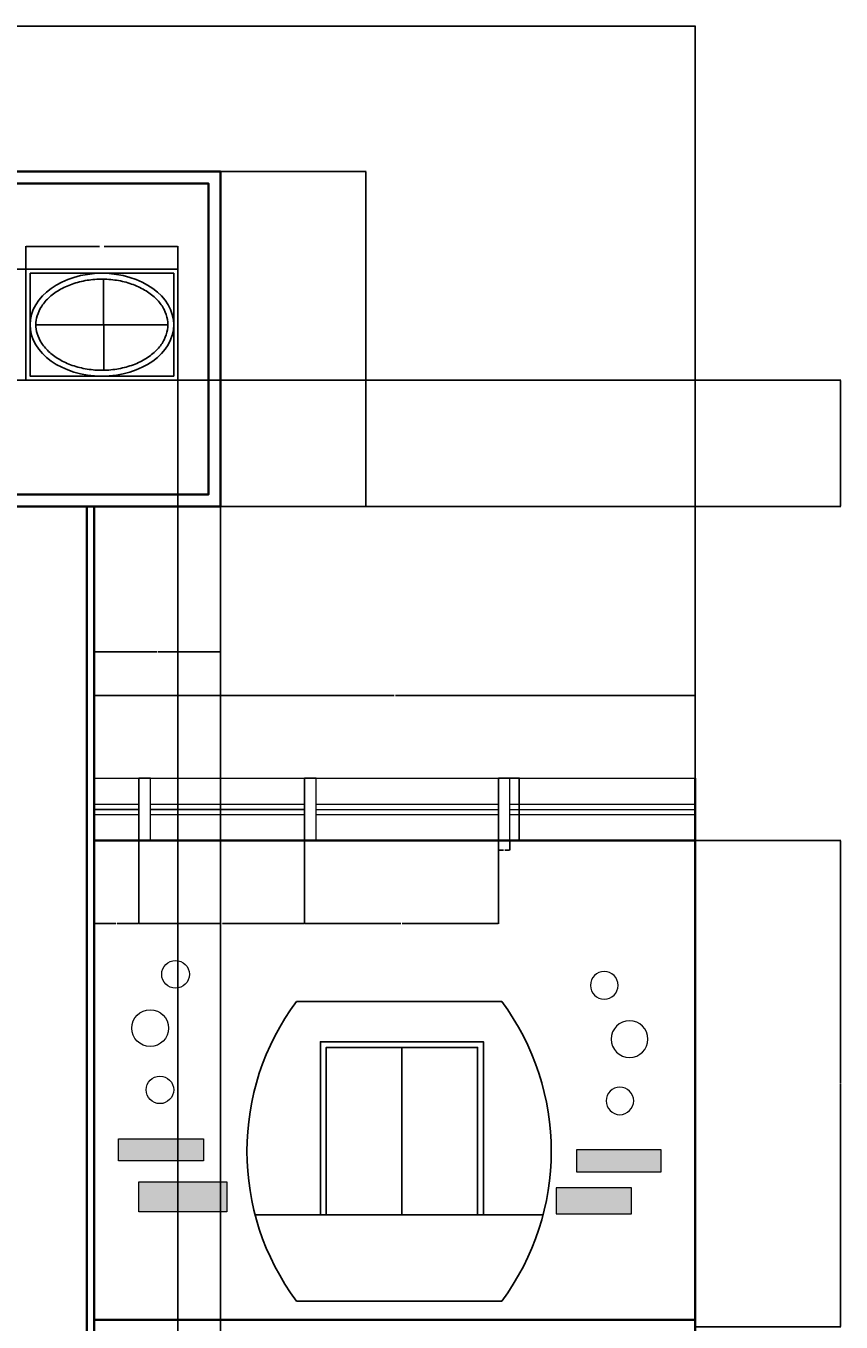
# Model space of a CAD drawing. Units: inches. Extents: x 328 to 2318, y 647 to 2548.
# Tile 5 of 5: x 1799 to 2318, y 1724 to 2548. Entities that reach past the tile are written whole.
import ezdxf

# ---------------------------------------------------------------- set-up
doc = ezdxf.new("R2010")
doc.units = ezdxf.units.IN
doc.header["$MEASUREMENT"] = 0
for name, color, linetype, lineweight in [('A-ANNO-DIMS', 2, 'Continuous', 18), ('A-ELEV', 7, 'Continuous', 35), ('A-ELEV-ORNM', 7, 'Continuous', 18), ('A-GLAZ', 4, 'Continuous', 25), ('A-ROOF', 7, 'Continuous', 35), ('A-ROOF-HRAL', 8, 'Continuous', 18)]:
    doc.layers.add(name, color=color, linetype=linetype, lineweight=lineweight)
doc.layers.add('A-ELEV-ORNM-PATT', color=18, linetype='Continuous', lineweight=13, true_color=0x000000)
doc.styles.get("Standard").update_dxf_attribs({"font": 'arial.ttf'})
doc.dimstyles.get("Standard").update_dxf_attribs({"dimtxt": 0.18, "dimasz": 0.18, "dimexe": 0.18, "dimexo": 0.0625, "dimgap": 0.09, "dimtad": 0, "dimtih": 1, "dimtoh": 1, "dimdec": 4, "dimzin": 0, "dimdsep": 46, "dimtxsty": 'Standard', "dimcen": 0.09, "dimadec": 0, "dimazin": 0, "dimtfac": 1, "dimtdec": 4, "dimtofl": 0, "dimtmove": 0, "dimatfit": 3, "dimfxl": 1, "dimtolj": 1, "dimtzin": 0, "dimarcsym": 0})

# ---------------------------------------------------------------- blocks, each defined once
blk = doc.blocks.new('WIN-ELEV-CURVED-SURROUND')
for p, q in [((162.11, 190.69), (31.57, 190.69)), ((98.64, 161.37), (98.64, 54.8)), ((5.23, 54.8), (188.45, 54.8)), ((31.57, 0), (162.11, 0))]:
    blk.add_line(p, q)
for points in [[(150.48, 54.8), (150.48, 165.07), (46.8, 165.07), (46.8, 54.8)], [(146.78, 54.8), (146.78, 161.37), (50.49, 161.37), (50.49, 54.8)]]:
    blk.add_lwpolyline(points)
for centre, start, end in [((159.76, 95.35), 143.35881, 216.64119), ((33.92, 95.35), 323.35881, 36.64119)]:
    blk.add_arc(centre, 159.76, start, end)
blk = doc.blocks.new('WIN-ELEV-OVAL')
for p, q in [((49.54, 6.37), (49.37, 64.33)), ((6.36, 35.36), (90.36, 35.36))]:
    blk.add_line(p, q)
for points in [[(0, 70.7), (96.72, 70.7), (96.72, 0), (0, 0)], [(2.67, 68.03), (94.06, 68.03), (94.06, 2.67), (2.67, 2.67)]]:
    blk.add_lwpolyline(points, close=True)
blk.add_ellipse((48.36, 35.35), major_axis=(-45.7, 0), ratio=0.715242)
blk.add_open_spline([(6.36, 35.35), (6.36, 33.47), (6.63, 31.58), (7.79, 27.59), (8.77, 25.48), (11.44, 21.43), (13.14, 19.48), (17.17, 15.88), (19.51, 14.22), (24.72, 11.33), (27.59, 10.09), (33.68, 8.11), (36.9, 7.38), (43.51, 6.46), (46.9, 6.28), (53.63, 6.5), (56.98, 6.89), (63.44, 8.21), (66.55, 9.15), (72.35, 11.49), (75.04, 12.9), (79.83, 16.09), (81.94, 17.87), (85.48, 21.67), (86.9, 23.7), (89.04, 27.86), (89.75, 29.99), (90.45, 34.29), (90.45, 36.45), (89.74, 40.75), (89.02, 42.88), (86.88, 47.04), (85.45, 49.06), (81.9, 52.86), (79.79, 54.64), (74.99, 57.83), (72.3, 59.23), (66.49, 61.57), (63.38, 62.5), (56.92, 63.82), (53.57, 64.21), (46.83, 64.41), (43.45, 64.23), (36.84, 63.31), (33.62, 62.57), (27.53, 60.59), (24.67, 59.35), (19.47, 56.45), (17.13, 54.79), (13.1, 51.18), (11.41, 49.23), (8.75, 45.18), (7.78, 43.07), (6.63, 39.09), (6.36, 37.22), (6.36, 35.35)], degree=3, knots=[0, 0, 0, 0, 0.205219, 0.205219, 0.440189, 0.440189, 0.675159, 0.675159, 0.910128, 0.910128, 1.145098, 1.145098, 1.380068, 1.380068, 1.615038, 1.615038, 1.850008, 1.850008, 2.084978, 2.084978, 2.319948, 2.319948, 2.554918, 2.554918, 2.789887, 2.789887, 3.024857, 3.024857, 3.259827, 3.259827, 3.494797, 3.494797, 3.729767, 3.729767, 3.964737, 3.964737, 4.199707, 4.199707, 4.434676, 4.434676, 4.669646, 4.669646, 4.904616, 4.904616, 5.139586, 5.139586, 5.374556, 5.374556, 5.609526, 5.609526, 5.844496, 5.844496, 6.079466, 6.079466, 6.283185, 6.283185, 6.283185, 6.283185])
blk = doc.blocks.new('FACADE-THREE-ROUNDELS')
for centre, radius in [((27.83, 82.27), 8.8), ((11.7, 48.09), 11.7), ((17.88, 8.77), 8.77)]:
    blk.add_circle(centre, radius)
blk = doc.blocks.new('POST-PARAPET')
blk.add_lwpolyline([(0, 0), (7.34, 0), (7.34, 39.76), (0, 39.76)], close=True)
blk = doc.blocks.new('*D7')
at = {"layer": 'A-ANNO-DIMS', "color": 0, "lineweight": -2, "transparency": 16777216}
for p, q in [((1799.05, 2393.5), (1799.05, 2408.12)), ((1799.23, 2407.94), (1845.92, 2407.94)), ((1895.59, 2407.94), (1848.89, 2407.94)), ((1895.77, 2393.5), (1895.77, 2408.12))]:
    blk.add_line(p, q, dxfattribs=at)
at = {"layer": 'A-ANNO-DIMS', "color": 0, "transparency": 16777216}
for points in [[(1799.23, 2407.97), (1799.23, 2407.91), (1799.05, 2407.94)], [(1895.59, 2407.97), (1895.59, 2407.91), (1895.77, 2407.94)]]:
    blk.add_solid(points, dxfattribs=at)
at = {"layer": 'Defpoints', "color": 0, "transparency": 16777216}
for p in [(1895.77, 2407.94), (1799.05, 2393.44), (1895.77, 2393.44)]:
    blk.add_point(p, dxfattribs=at)
at = {"layer": 'A-ANNO-DIMS', "color": 0, "transparency": 16777216, "insert": (1847.41, 2407.94), "char_height": 0.18, "attachment_point": 5}
blk.add_mtext('\\A1;OVAL WINDOW 97 TYP.', dxfattribs=at)
blk = doc.blocks.new('*D8')
at = {"layer": 'A-ANNO-DIMS', "color": 0, "lineweight": -2, "transparency": 16777216}
for p, q in [((1798.98, 2393.44), (1784.36, 2393.44)), ((1784.54, 2393.26), (1784.54, 2358.27)), ((1784.54, 2322.92), (1784.54, 2357.91)), ((1798.98, 2322.74), (1784.36, 2322.74))]:
    blk.add_line(p, q, dxfattribs=at)
at = {"layer": 'A-ANNO-DIMS', "color": 0, "transparency": 16777216}
for points in [[(1784.51, 2393.26), (1784.57, 2393.26), (1784.54, 2393.44)], [(1784.51, 2322.92), (1784.57, 2322.92), (1784.54, 2322.74)]]:
    blk.add_solid(points, dxfattribs=at)
at = {"layer": 'Defpoints', "color": 0, "transparency": 16777216}
for p in [(1784.54, 2393.44), (1799.05, 2393.44), (1799.05, 2322.74)]:
    blk.add_point(p, dxfattribs=at)
at = {"layer": 'A-ANNO-DIMS', "color": 0, "transparency": 16777216, "insert": (1784.54, 2358.09), "char_height": 0.18, "attachment_point": 5}
blk.add_mtext('\\A1;71 TYP.', dxfattribs=at)
blk = doc.blocks.new('*D9')
at = {"layer": 'A-ANNO-DIMS', "color": 0, "lineweight": -2, "transparency": 16777216}
for p, q in [((2107.09, 2069.59), (2113.17, 2069.59)), ((2112.99, 2069.41), (2112.99, 2049.9)), ((2112.99, 2030.01), (2112.99, 2049.53)), ((2107.09, 2029.83), (2113.17, 2029.83))]:
    blk.add_line(p, q, dxfattribs=at)
at = {"layer": 'A-ANNO-DIMS', "color": 0, "transparency": 16777216}
for points in [[(2112.96, 2069.41), (2113.02, 2069.41), (2112.99, 2069.59)], [(2112.96, 2030.01), (2113.02, 2030.01), (2112.99, 2029.83)]]:
    blk.add_solid(points, dxfattribs=at)
at = {"layer": 'Defpoints', "color": 0, "transparency": 16777216}
for p in [(2107.02, 2069.59), (2112.99, 2069.59), (2107.02, 2029.83)]:
    blk.add_point(p, dxfattribs=at)
at = {"layer": 'A-ANNO-DIMS', "color": 0, "transparency": 16777216, "insert": (2112.99, 2049.71), "char_height": 0.18, "attachment_point": 5}
blk.add_mtext('\\A1;POST 40 TYP.', dxfattribs=at)
blk = doc.blocks.new('*D10')
at = {"layer": 'A-ANNO-DIMS', "color": 0, "lineweight": -2, "transparency": 16777216}
for p, q in [((2099.69, 2029.77), (2099.69, 2023.69)), ((2107.02, 2029.77), (2107.02, 2023.69)), ((2099.87, 2023.87), (2102.9, 2023.87)), ((2106.84, 2023.87), (2103.81, 2023.87))]:
    blk.add_line(p, q, dxfattribs=at)
at = {"layer": 'A-ANNO-DIMS', "color": 0, "transparency": 16777216}
for points in [[(2099.87, 2023.9), (2099.87, 2023.84), (2099.69, 2023.87)], [(2106.84, 2023.9), (2106.84, 2023.84), (2107.02, 2023.87)]]:
    blk.add_solid(points, dxfattribs=at)
at = {"layer": 'Defpoints', "color": 0, "transparency": 16777216}
for p in [(2099.69, 2029.83), (2107.02, 2029.83), (2107.02, 2023.87)]:
    blk.add_point(p, dxfattribs=at)
at = {"layer": 'A-ANNO-DIMS', "color": 0, "transparency": 16777216, "insert": (2103.35, 2023.87), "char_height": 0.18, "attachment_point": 5}
blk.add_mtext('\\A1;7 TYP.', dxfattribs=at)
blk = doc.blocks.new('*D39')
at = {"layer": 'A-ANNO-DIMS', "color": 0, "lineweight": -2, "transparency": 16777216}
for p, q in [((1060.28, 1725.1), (1060.28, 2548.17)), ((2224.98, 2069.65), (2224.98, 2548.17)), ((1060.46, 2547.99), (1642.17, 2547.99)), ((2224.8, 2547.99), (1643.08, 2547.99))]:
    blk.add_line(p, q, dxfattribs=at)
at = {"layer": 'A-ANNO-DIMS', "color": 0, "transparency": 16777216}
for points in [[(1060.46, 2548.02), (1060.46, 2547.96), (1060.28, 2547.99)], [(2224.8, 2548.02), (2224.8, 2547.96), (2224.98, 2547.99)]]:
    blk.add_solid(points, dxfattribs=at)
at = {"layer": 'Defpoints', "color": 0, "transparency": 16777216}
for p in [(2224.98, 2547.99), (2224.98, 2069.59), (1060.28, 1725.04)]:
    blk.add_point(p, dxfattribs=at)
at = {"layer": 'A-ANNO-DIMS', "color": 0, "transparency": 16777216, "insert": (1642.63, 2547.99), "char_height": 0.18, "attachment_point": 5}
blk.add_mtext('\\A1;1164.7', dxfattribs=at)
blk = doc.blocks.new('*D42')
at = {"layer": 'A-ANNO-DIMS', "color": 0, "lineweight": -2, "transparency": 16777216}
for p, q in [((1842.45, 2029.9), (1842.45, 2122.46)), ((1842.63, 2122.28), (2033.32, 2122.28)), ((2224.8, 2122.28), (2034.11, 2122.28)), ((2224.98, 2029.9), (2224.98, 2122.46))]:
    blk.add_line(p, q, dxfattribs=at)
at = {"layer": 'A-ANNO-DIMS', "color": 0, "transparency": 16777216}
for points in [[(1842.63, 2122.31), (1842.63, 2122.25), (1842.45, 2122.28)], [(2224.8, 2122.31), (2224.8, 2122.25), (2224.98, 2122.28)]]:
    blk.add_solid(points, dxfattribs=at)
at = {"layer": 'Defpoints', "color": 0, "transparency": 16777216}
for p in [(2224.98, 2122.28), (1842.45, 2029.83), (2224.98, 2029.83)]:
    blk.add_point(p, dxfattribs=at)
at = {"layer": 'A-ANNO-DIMS', "color": 0, "transparency": 16777216, "insert": (2033.72, 2122.28), "char_height": 0.18, "attachment_point": 5}
blk.add_mtext('\\A1;382.5', dxfattribs=at)
blk = doc.blocks.new('*D46')
at = {"layer": 'A-ANNO-DIMS', "color": 0, "lineweight": -2, "transparency": 16777216}
for p, q in [((2225.04, 2029.83), (2317.61, 2029.83)), ((2317.43, 2029.65), (2317.43, 1875.33)), ((2317.43, 1720.64), (2317.43, 1874.96)), ((2225.04, 1720.46), (2317.61, 1720.46))]:
    blk.add_line(p, q, dxfattribs=at)
at = {"layer": 'A-ANNO-DIMS', "color": 0, "transparency": 16777216}
for points in [[(2317.4, 2029.65), (2317.46, 2029.65), (2317.43, 2029.83)], [(2317.4, 1720.64), (2317.46, 1720.64), (2317.43, 1720.46)]]:
    blk.add_solid(points, dxfattribs=at)
at = {"layer": 'Defpoints', "color": 0, "transparency": 16777216}
for p in [(2224.98, 2029.83), (2317.43, 2029.83), (2224.98, 1720.46)]:
    blk.add_point(p, dxfattribs=at)
at = {"layer": 'A-ANNO-DIMS', "color": 0, "transparency": 16777216, "insert": (2317.43, 1875.15), "char_height": 0.18, "attachment_point": 5}
blk.add_mtext('\\A1;309.4', dxfattribs=at)
blk = doc.blocks.new('*D48')
at = {"layer": 'A-ANNO-DIMS', "color": 0, "lineweight": -2, "transparency": 16777216}
for p, q in [((1842.45, 2242.37), (1842.45, 2149.8)), ((1922.92, 2242.37), (1922.92, 2149.8)), ((1842.63, 2149.98), (1882.29, 2149.98)), ((1922.74, 2149.98), (1883.08, 2149.98))]:
    blk.add_line(p, q, dxfattribs=at)
at = {"layer": 'A-ANNO-DIMS', "color": 0, "transparency": 16777216}
for points in [[(1842.63, 2150.01), (1842.63, 2149.95), (1842.45, 2149.98)], [(1922.74, 2150.01), (1922.74, 2149.95), (1922.92, 2149.98)]]:
    blk.add_solid(points, dxfattribs=at)
at = {"layer": 'Defpoints', "color": 0, "transparency": 16777216}
for p in [(1842.45, 2242.43), (1922.92, 2242.43), (1842.45, 2149.98)]:
    blk.add_point(p, dxfattribs=at)
at = {"layer": 'A-ANNO-DIMS', "color": 0, "transparency": 16777216, "insert": (1882.69, 2149.98), "char_height": 0.18, "attachment_point": 5}
blk.add_mtext('\\A1;80.47', dxfattribs=at)
blk = doc.blocks.new('*D49')
at = {"layer": 'A-ANNO-DIMS', "color": 0, "lineweight": -2, "transparency": 16777216}
for p, q in [((1922.99, 2455.54), (2015.55, 2455.54)), ((2015.37, 2455.36), (2015.37, 2349.17)), ((2015.37, 2242.61), (2015.37, 2348.8)), ((1922.99, 2242.43), (2015.55, 2242.43))]:
    blk.add_line(p, q, dxfattribs=at)
at = {"layer": 'A-ANNO-DIMS', "color": 0, "transparency": 16777216}
for points in [[(2015.34, 2455.36), (2015.4, 2455.36), (2015.37, 2455.54)], [(2015.34, 2242.61), (2015.4, 2242.61), (2015.37, 2242.43)]]:
    blk.add_solid(points, dxfattribs=at)
at = {"layer": 'Defpoints', "color": 0, "transparency": 16777216}
for p in [(1922.92, 2455.54), (1922.92, 2242.43), (2015.37, 2242.43)]:
    blk.add_point(p, dxfattribs=at)
at = {"layer": 'A-ANNO-DIMS', "color": 0, "transparency": 16777216, "insert": (2015.37, 2348.98), "char_height": 0.18, "attachment_point": 5}
blk.add_mtext('\\A1;213.1', dxfattribs=at)
blk = doc.blocks.new('*D60')
at = {"layer": 'A-ANNO-DIMS', "color": 0, "lineweight": -2, "transparency": 16777216}
for p, q in [((1895.83, 2322.74), (2317.61, 2322.74)), ((2317.43, 2322.56), (2317.43, 2282.76)), ((2317.43, 2242.61), (2317.43, 2282.4)), ((1922.99, 2242.43), (2317.61, 2242.43))]:
    blk.add_line(p, q, dxfattribs=at)
at = {"layer": 'A-ANNO-DIMS', "color": 0, "transparency": 16777216}
for points in [[(2317.4, 2322.56), (2317.46, 2322.56), (2317.43, 2322.74)], [(2317.4, 2242.61), (2317.46, 2242.61), (2317.43, 2242.43)]]:
    blk.add_solid(points, dxfattribs=at)
at = {"layer": 'Defpoints', "color": 0, "transparency": 16777216}
for p in [(1895.77, 2322.74), (2317.43, 2322.74), (1922.92, 2242.43)]:
    blk.add_point(p, dxfattribs=at)
at = {"layer": 'A-ANNO-DIMS', "color": 0, "transparency": 16777216, "insert": (2317.43, 2282.58), "char_height": 0.18, "attachment_point": 5}
blk.add_mtext('\\A1;80.3', dxfattribs=at)
blk = doc.blocks.new('*D61')
at = {"layer": 'A-ANNO-DIMS', "color": 0, "lineweight": -2, "transparency": 16777216}
for p, q in [((1895.77, 2322.67), (1895.77, 696.16)), ((1922.92, 2242.37), (1922.92, 696.16)), ((1895.95, 696.34), (1908.88, 696.34)), ((1922.74, 696.34), (1909.81, 696.34))]:
    blk.add_line(p, q, dxfattribs=at)
at = {"layer": 'A-ANNO-DIMS', "color": 0, "transparency": 16777216}
for points in [[(1895.95, 696.37), (1895.95, 696.31), (1895.77, 696.34)], [(1922.74, 696.37), (1922.74, 696.31), (1922.92, 696.34)]]:
    blk.add_solid(points, dxfattribs=at)
at = {"layer": 'Defpoints', "color": 0, "transparency": 16777216}
for p in [(1895.77, 2322.74), (1922.92, 2242.43), (1895.77, 696.34)]:
    blk.add_point(p, dxfattribs=at)
at = {"layer": 'A-ANNO-DIMS', "color": 0, "transparency": 16777216, "insert": (1909.35, 696.34), "char_height": 0.18, "attachment_point": 5}
blk.add_mtext('\\A1;27.154', dxfattribs=at)
blk = doc.blocks.new('*D65')
at = {"layer": 'A-ANNO-DIMS', "color": 0, "lineweight": -2, "transparency": 16777216}
for p, q in [((1842.45, 2069.53), (1842.45, 1976.96)), ((1870.93, 2069.53), (1870.93, 1976.96)), ((1842.63, 1977.14), (1856.3, 1977.14)), ((1870.75, 1977.14), (1857.09, 1977.14))]:
    blk.add_line(p, q, dxfattribs=at)
at = {"layer": 'A-ANNO-DIMS', "color": 0, "transparency": 16777216}
for points in [[(1842.63, 1977.17), (1842.63, 1977.11), (1842.45, 1977.14)], [(1870.75, 1977.17), (1870.75, 1977.11), (1870.93, 1977.14)]]:
    blk.add_solid(points, dxfattribs=at)
at = {"layer": 'Defpoints', "color": 0, "transparency": 16777216}
for p in [(1842.45, 2069.59), (1870.93, 2069.59), (1842.45, 1977.14)]:
    blk.add_point(p, dxfattribs=at)
at = {"layer": 'A-ANNO-DIMS', "color": 0, "transparency": 16777216, "insert": (1856.69, 1977.14), "char_height": 0.18, "attachment_point": 5}
blk.add_mtext('\\A1;28.48', dxfattribs=at)
blk = doc.blocks.new('*D66')
at = {"layer": 'A-ANNO-DIMS', "color": 0, "lineweight": -2, "transparency": 16777216}
for p, q in [((1870.93, 2069.53), (1870.93, 1976.96)), ((1976.3, 2069.53), (1976.3, 1976.96)), ((1871.11, 1977.14), (1923.16, 1977.14)), ((1976.12, 1977.14), (1924.07, 1977.14))]:
    blk.add_line(p, q, dxfattribs=at)
at = {"layer": 'A-ANNO-DIMS', "color": 0, "transparency": 16777216}
for points in [[(1871.11, 1977.17), (1871.11, 1977.11), (1870.93, 1977.14)], [(1976.12, 1977.17), (1976.12, 1977.11), (1976.3, 1977.14)]]:
    blk.add_solid(points, dxfattribs=at)
at = {"layer": 'Defpoints', "color": 0, "transparency": 16777216}
for p in [(1870.93, 2069.59), (1976.3, 2069.59), (1870.93, 1977.14)]:
    blk.add_point(p, dxfattribs=at)
at = {"layer": 'A-ANNO-DIMS', "color": 0, "transparency": 16777216, "insert": (1923.62, 1977.14), "char_height": 0.18, "attachment_point": 5}
blk.add_mtext('\\A1;105.37', dxfattribs=at)
blk = doc.blocks.new('*D67')
at = {"layer": 'A-ANNO-DIMS', "color": 0, "lineweight": -2, "transparency": 16777216}
for p, q in [((1976.3, 2069.53), (1976.3, 1976.96)), ((2099.69, 2069.53), (2099.69, 1976.96)), ((1976.48, 1977.14), (2037.54, 1977.14)), ((2099.51, 1977.14), (2038.45, 1977.14))]:
    blk.add_line(p, q, dxfattribs=at)
at = {"layer": 'A-ANNO-DIMS', "color": 0, "transparency": 16777216}
for points in [[(1976.48, 1977.17), (1976.48, 1977.11), (1976.3, 1977.14)], [(2099.51, 1977.17), (2099.51, 1977.11), (2099.69, 1977.14)]]:
    blk.add_solid(points, dxfattribs=at)
at = {"layer": 'Defpoints', "color": 0, "transparency": 16777216}
for p in [(1976.3, 2069.59), (2099.69, 2069.59), (1976.3, 1977.14)]:
    blk.add_point(p, dxfattribs=at)
at = {"layer": 'A-ANNO-DIMS', "color": 0, "transparency": 16777216, "insert": (2037.99, 1977.14), "char_height": 0.18, "attachment_point": 5}
blk.add_mtext('\\A1;123.39', dxfattribs=at)

msp = doc.modelspace()

# ---------------------------------------------------------------- hatches: boundary and pattern name
at = {"layer": 'A-ELEV-ORNM-PATT'}
h = msp.add_hatch(color=256, dxfattribs=at)
h.dxf.hatch_style = 1
h.paths.add_polyline_path([(1160.8736, 1194.017), (1104.946, 1194.017), (1104.946, 1174.8467), (1160.8736, 1174.8467)])
h.paths.add_polyline_path([(1145.9162, 1221.3103), (1091.9395, 1221.3103), (1091.9395, 1207.3388), (1145.9162, 1207.3388)])
h.paths.add_polyline_path([(1418.337, 1190.1501), (1370.4156, 1190.1501), (1370.4156, 1173.7241), (1418.337, 1173.7241)])
h.paths.add_polyline_path([(1437.3105, 1214.299), (1383.3339, 1214.299), (1383.3339, 1200.3274), (1437.3105, 1200.3274)])
h.paths.add_polyline_path([(1418.337, 1499.5227), (1370.4156, 1499.5227), (1370.4156, 1483.0967), (1418.337, 1483.0967)])
h.paths.add_polyline_path([(1437.3105, 1523.6716), (1383.3339, 1523.6716), (1383.3339, 1509.7), (1437.3105, 1509.7)])
h.paths.add_polyline_path([(1145.9162, 1530.683), (1091.9395, 1530.683), (1091.9395, 1516.7114), (1145.9162, 1516.7114)])
h.paths.add_polyline_path([(1160.8736, 1503.3896), (1104.946, 1503.3896), (1104.946, 1484.2194), (1160.8736, 1484.2194)])
h.paths.add_polyline_path([(1160.8736, 1812.7623), (1104.946, 1812.7623), (1104.946, 1793.592), (1160.8736, 1793.592)])
h.paths.add_polyline_path([(1145.9162, 1840.0556), (1091.9395, 1840.0556), (1091.9395, 1826.084), (1145.9162, 1826.084)])
h.paths.add_polyline_path([(1437.3105, 1833.0442), (1383.3339, 1833.0442), (1383.3339, 1819.0726), (1437.3105, 1819.0726)])
h.paths.add_polyline_path([(1418.337, 1808.8953), (1370.4156, 1808.8953), (1370.4156, 1792.4693), (1418.337, 1792.4693)])
h.paths.add_polyline_path([(1145.9162, 908.3867), (1091.9395, 908.3867), (1091.9395, 894.4151), (1145.9162, 894.4151)])
h.paths.add_polyline_path([(1160.8736, 881.0933), (1104.946, 881.0933), (1104.946, 861.923), (1160.8736, 861.923)])
h.paths.add_polyline_path([(1418.337, 877.2264), (1370.4156, 877.2264), (1370.4156, 860.8004), (1418.337, 860.8004)])
h.paths.add_polyline_path([(1437.3105, 901.3753), (1383.3339, 901.3753), (1383.3339, 887.4037), (1437.3105, 887.4037)])
h.paths.add_polyline_path([(1926.897, 881.0933), (1870.9694, 881.0933), (1870.9694, 861.923), (1926.897, 861.923)])
h.paths.add_polyline_path([(1911.9396, 908.3867), (1857.9629, 908.3867), (1857.9629, 894.4151), (1911.9396, 894.4151)])
h.paths.add_polyline_path([(2184.3603, 877.2264), (2136.439, 877.2264), (2136.439, 860.8004), (2184.3603, 860.8004)])
h.paths.add_polyline_path([(2203.3339, 901.3753), (2149.3572, 901.3753), (2149.3572, 887.4037), (2203.3339, 887.4037)])
h.paths.add_polyline_path([(2184.3603, 1190.1501), (2136.439, 1190.1501), (2136.439, 1173.7241), (2184.3603, 1173.7241)])
h.paths.add_polyline_path([(2203.3339, 1214.299), (2149.3572, 1214.299), (2149.3572, 1200.3274), (2203.3339, 1200.3274)])
h.paths.add_polyline_path([(1911.9396, 1221.3103), (1857.9629, 1221.3103), (1857.9629, 1207.3388), (1911.9396, 1207.3388)])
h.paths.add_polyline_path([(1926.897, 1194.017), (1870.9694, 1194.017), (1870.9694, 1174.8467), (1926.897, 1174.8467)])
h.paths.add_polyline_path([(1926.897, 1503.3896), (1870.9694, 1503.3896), (1870.9694, 1484.2194), (1926.897, 1484.2194)])
h.paths.add_polyline_path([(1911.9396, 1530.683), (1857.9629, 1530.683), (1857.9629, 1516.7114), (1911.9396, 1516.7114)])
h.paths.add_polyline_path([(2184.3603, 1499.5227), (2136.439, 1499.5227), (2136.439, 1483.0967), (2184.3603, 1483.0967)])
h.paths.add_polyline_path([(2203.3339, 1523.6716), (2149.3572, 1523.6716), (2149.3572, 1509.7), (2203.3339, 1509.7)])
h.paths.add_polyline_path([(1926.897, 1812.7623), (1870.9694, 1812.7623), (1870.9694, 1793.592), (1926.897, 1793.592)])
h.paths.add_polyline_path([(1911.9396, 1840.0556), (1857.9629, 1840.0556), (1857.9629, 1826.084), (1911.9396, 1826.084)])
h.paths.add_polyline_path([(2184.3603, 1808.8953), (2136.439, 1808.8953), (2136.439, 1792.4693), (2184.3603, 1792.4693)])
h.paths.add_polyline_path([(2203.3339, 1833.0442), (2149.3572, 1833.0442), (2149.3572, 1819.0726), (2203.3339, 1819.0726)])

# ---------------------------------------------------------------- linework, layer by layer
at = {"layer": 'A-ELEV'}
for p, q in [((1842.45, 2242.4288), (1442.8075, 2242.4288)), ((1837.8703, 1106.2944), (1837.8703, 2242.4288)), ((1842.45, 788.791), (1842.45, 2242.4288)), ((2224.9815, 788.791), (2224.9815, 2069.5914)), ((1842.45, 2029.8325), (2224.9815, 2029.8325)), ((1842.45, 1725.0396), (2224.9815, 1725.0396))]:
    msp.add_line(p, q, dxfattribs=at)
at = {"layer": 'A-ELEV-ORNM'}
for points in [[(1857.9629, 1840.0556), (1911.9396, 1840.0556), (1911.9396, 1826.084), (1857.9629, 1826.084)], [(2203.3339, 1833.0442), (2149.3572, 1833.0442), (2149.3572, 1819.0726), (2203.3339, 1819.0726)], [(1870.9694, 1812.7623), (1926.897, 1812.7623), (1926.897, 1793.592), (1870.9694, 1793.592)], [(2184.3603, 1808.8953), (2136.439, 1808.8953), (2136.439, 1792.4693), (2184.3603, 1792.4693)]]:
    msp.add_lwpolyline(points, close=True, dxfattribs=at)
at = {"layer": 'A-ROOF'}
for points in [[(1362.3871, 2242.4288), (1922.9232, 2242.4288), (1922.9232, 2455.5387), (1362.3871, 2455.5387)], [(1370.0417, 2250.0835), (1915.2686, 2250.0835), (1915.2686, 2447.8841), (1370.0417, 2447.8841)]]:
    msp.add_lwpolyline(points, close=True, dxfattribs=at)
at = {"layer": 'A-ROOF-HRAL'}
for p, q in [((1842.45, 2069.5914), (2224.9815, 2069.5914)), ((1842.45, 2053.0614), (1870.9325, 2053.0614)), ((1842.45, 2049.712), (1870.9325, 2049.712)), ((1870.9325, 2049.712), (1842.45, 2049.712)), ((1842.45, 2046.4313), (1870.9325, 2046.4313)), ((1878.2688, 2053.0614), (1976.299, 2053.0614)), ((1976.299, 2049.712), (1878.2688, 2049.712)), ((1878.2688, 2049.712), (1976.299, 2049.712)), ((1878.2688, 2046.4313), (1976.299, 2046.4313)), ((1905.5419, 2053.0614), (1976.299, 2053.0614)), ((1905.5419, 2049.712), (1976.299, 2049.712)), ((1905.5419, 2046.4313), (1976.299, 2046.4313)), ((1983.6352, 2053.0614), (2099.6863, 2053.0614)), ((1983.6352, 2049.712), (2099.6863, 2049.712)), ((1983.6352, 2046.4313), (2099.6863, 2046.4313)), ((2019.7781, 2053.0614), (2099.6863, 2053.0614)), ((2019.7781, 2049.712), (2099.6863, 2049.712)), ((2019.7781, 2046.4313), (2099.6863, 2046.4313)), ((2107.0226, 2053.0614), (2224.9815, 2053.0614)), ((2107.0226, 2049.712), (2224.9815, 2049.712)), ((2107.0226, 2046.4313), (2224.9815, 2046.4313)), ((2118.2938, 2053.0614), (2208.8309, 2053.0614)), ((2118.2938, 2049.712), (2208.8309, 2049.712)), ((2118.2938, 2046.4313), (2208.8309, 2046.4313))]:
    msp.add_line(p, q, dxfattribs=at)

# ---------------------------------------------------------------- block references
at = {"layer": 'A-ELEV-ORNM'}
msp.add_blockref('FACADE-THREE-ROUNDELS', (1866.4251, 1862.5181), dxfattribs=at)
at = {"layer": 'A-ELEV-ORNM', "extrusion": (0, 0, -1), "zscale": -1}
msp.add_blockref('FACADE-THREE-ROUNDELS', (-2194.8717, 1855.5067), dxfattribs=at)
at = {"layer": 'A-GLAZ'}
for name, p in [('WIN-ELEV-OVAL', (1799.0469, 2322.7365)), ('WIN-ELEV-CURVED-SURROUND', (1939.6727, 1736.8753))]:
    msp.add_blockref(name, p, dxfattribs=at)
at = {"layer": 'A-ROOF-HRAL'}
for p in [(1870.9325, 2029.8325), (1976.299, 2029.8325), (2099.6863, 2029.8325)]:
    msp.add_blockref('POST-PARAPET', p, dxfattribs=at)

# ---------------------------------------------------------------- dimensions: what is measured, and where the dimension line sits
at = {"layer": 'A-ANNO-DIMS'}
for base, p1, p2, override, picture, middle in [((2224.9815, 2547.9887), (1060.276, 1725.0396), (2224.9815, 2069.5914), {"dimdec": 1, "dimlfac": 1, "dimrnd": 0, "dimzin": 0, "dimdsep": 46, "dimlunit": 2}, '*D39', (1642.6287, 2547.9887)), ((1895.76968, 696.34097), (1922.92323, 2242.42884), (1895.76968, 2322.73649), {"dimdec": 3, "dimlfac": 1, "dimrnd": 0, "dimzin": 0, "dimdsep": 46, "dimlunit": 2}, '*D61', (1909.34646, 696.34097)), ((2224.9815, 2122.2825), (1842.45, 2029.8325), (2224.9815, 2029.8325), {"dimdec": 1, "dimlfac": 1, "dimrnd": 0, "dimzin": 0, "dimdsep": 46, "dimlunit": 2}, '*D42', (2033.7157, 2122.2825))]:
    dim = msp.add_linear_dim(base=base, p1=p1, p2=p2, dimstyle='Standard', override=override, dxfattribs=at)
    dim.commit()
    dim.dimension.update_dxf_attribs({"geometry": picture, "text_midpoint": middle})
for base, p1, p2, angle, override, picture, middle in [((2015.3732, 2242.4288), (1922.9232, 2455.5387), (1922.9232, 2242.4288), 270, {"dimdec": 1, "dimlfac": 1, "dimrnd": 0, "dimzin": 0, "dimdsep": 46, "dimlunit": 2}, '*D49', (2015.3732, 2348.9838)), ((2317.4315, 2322.7365), (1922.9232, 2242.4288), (1895.7697, 2322.7365), 90, {"dimdec": 1, "dimlfac": 1, "dimrnd": 0, "dimzin": 0, "dimdsep": 46, "dimlunit": 2}, '*D60', (2317.4315, 2282.5827)), ((1842.45, 2149.9788), (1922.9232, 2242.4288), (1842.45, 2242.4288), 180, {"dimdec": 2, "dimlfac": 1, "dimrnd": 0, "dimzin": 0, "dimdsep": 46, "dimlunit": 2}, '*D48', (1882.6866, 2149.9788)), ((1842.45, 1977.1414), (1870.9325, 2069.5914), (1842.45, 2069.5914), 180, {"dimdec": 2, "dimlfac": 1, "dimrnd": 0, "dimzin": 0, "dimdsep": 46, "dimlunit": 2}, '*D65', (1856.6913, 1977.1414)), ((1870.9325, 1977.1414), (1976.299, 2069.5914), (1870.9325, 2069.5914), 180, {"dimdec": 2, "dimlfac": 1, "dimrnd": 0, "dimzin": 0, "dimdsep": 46, "dimlunit": 2}, '*D66', (1923.6157, 1977.1414)), ((1976.299, 1977.1414), (2099.6863, 2069.5914), (1976.299, 2069.5914), 180, {"dimdec": 2, "dimlfac": 1, "dimrnd": 0, "dimzin": 0, "dimdsep": 46, "dimlunit": 2}, '*D67', (2037.9926, 1977.1414)), ((2317.4315, 2029.8325), (2224.9815, 1720.4599), (2224.9815, 2029.8325), 90, {"dimdec": 1, "dimlfac": 1, "dimrnd": 0, "dimzin": 0, "dimdsep": 46, "dimlunit": 2}, '*D46', (2317.4315, 1875.1462))]:
    dim = msp.add_linear_dim(base=base, p1=p1, p2=p2, angle=angle, dimstyle='Standard', override=override, dxfattribs=at)
    dim.commit()
    dim.dimension.update_dxf_attribs({"geometry": picture, "text_midpoint": middle})
for base, p1, p2, text, picture, middle in [((1895.7697, 2407.9435), (1799.0469, 2393.4351), (1895.7697, 2393.4351), 'OVAL WINDOW <> TYP.', '*D7', (1847.4083, 2407.9435)), ((2107.0226, 2023.8687), (2099.6863, 2029.8325), (2107.0226, 2029.8325), '<> TYP.', '*D10', (2103.3545, 2023.8687))]:
    dim = msp.add_linear_dim(base=base, p1=p1, p2=p2, text=text, dimstyle='Standard', override={"dimdec": 0, "dimlfac": 1, "dimrnd": 0, "dimzin": 0, "dimdsep": 46, "dimlunit": 2}, dxfattribs=at)
    dim.commit()
    dim.dimension.update_dxf_attribs({"geometry": picture, "text_midpoint": middle})
for base, p1, p2, text, picture, middle in [((1784.5385, 2393.4351), (1799.0469, 2322.7365), (1799.0469, 2393.4351), '<> TYP.', '*D8', (1784.5385, 2358.0858)), ((2112.9864, 2069.5914), (2107.0226, 2029.8325), (2107.0226, 2069.5914), 'POST <> TYP.', '*D9', (2112.9864, 2049.712))]:
    dim = msp.add_linear_dim(base=base, p1=p1, p2=p2, angle=90, text=text, dimstyle='Standard', override={"dimdec": 0, "dimlfac": 1, "dimrnd": 0, "dimzin": 0, "dimdsep": 46, "dimlunit": 2}, dxfattribs=at)
    dim.commit()
    dim.dimension.update_dxf_attribs({"geometry": picture, "text_midpoint": middle})

doc.saveas('drawing.dxf')
